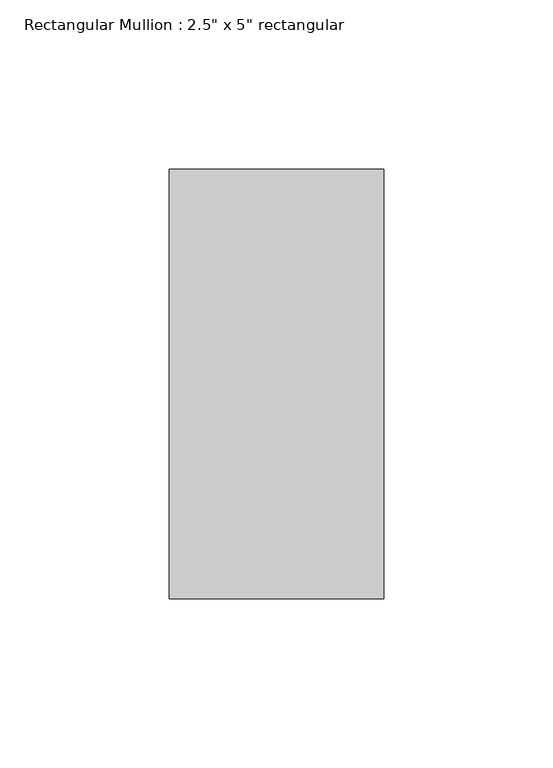
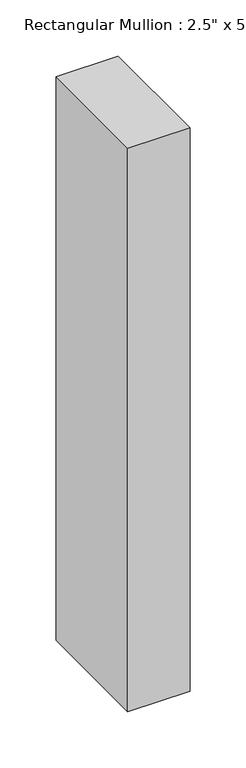
"""IFC4 building model written with IfcOpenShell, lengths in millimetres: member geometry."""

from ifc_helpers import new_model, si_unit, frame, origin, place, context, project, spatial, polyline, outline, extrude, source, transform, mapped, element, save


def member_6b5d0785(model_context):
    return source(origin(), model_context, "Body", "SweptSolid", [
        extrude(outline(polyline([(0.0, 63.5), (0.0, -63.5), (-63.5, -63.5), (-63.5, 63.5), (0.0, 63.5)])), frame((0.0, 0.0, -610.0265622), z_axis=(0.0, 0.0, 1.0), x_axis=(1.0, 0.0, 0.0)), (0.0, 0.0, 1.0), 610.0265622),
    ])


if __name__ == "__main__":
    model = new_model("IFC4")
    model_context = context("Model", 3, world=origin())
    ifc_project = project(units=[si_unit("LENGTHUNIT", "METRE", prefix="MILLI")], contexts=[model_context])
    site = spatial("IfcSite", under=ifc_project)
    building = spatial("IfcBuilding", under=site)
    placement = place(None, origin())
    member_shape = member_6b5d0785(model_context)
    element("IfcMember", 1, ObjectType="Rectangular Mullion : 2.5\" x 5\" rectangular", at=placement, inside=building, context=model_context, shape_type="MappedRepresentation", body=[
        mapped(member_shape, transform((0.0, 0.0, 0.0), x_axis=(1.0, 0.0, 0.0), y_axis=(0.0, 1.0, 0.0), z_axis=(0.0, 0.0, 1.0))),
    ])
    save(model, "model.ifc")

# Revit data of these elements
# Type "Rectangular Mullion : 2.5\" x 5\" rectangular"
#   built-in parameter 1007304 = 0.416667 (stored number, unit not read)
#   built-in parameter 1007301 = 0.104167 (stored number, unit not read)
#   built-in parameter 1007300 = 0.104167 (stored number, unit not read)
# Element 1 (IfcMember, "Rectangular Mullion : 2.5\" x 5\" rectangular")
#   Materials on its faces: "Aluminum"
# Materials
#   "Aluminum": class "Metal", colour RGB 247 247 247, transparency 0, Description = "Aluminum 6061", Cost = 0
